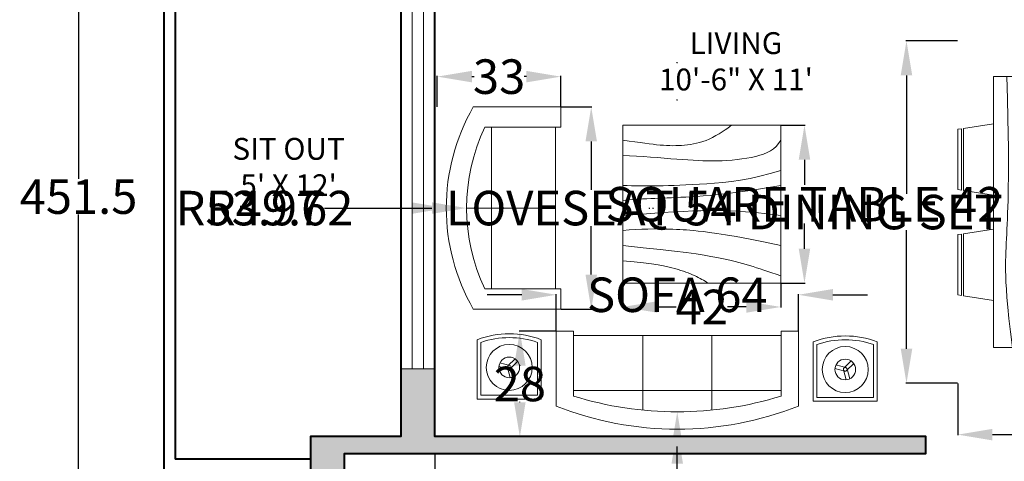
# Model space of a CAD drawing. Units: inches. Extents: x -51 to 563, y -59 to 453.
# Tile 2 of 6: x -51 to 211, y 125 to 242. Entities that reach past the tile are written whole.
import ezdxf

# ---------------------------------------------------------------- set-up
doc = ezdxf.new("R2010")
doc.units = ezdxf.units.IN
doc.header["$MEASUREMENT"] = 0
for name, color, linetype, lineweight in [('A-ANNO-DIMS', 2, 'Continuous', 18), ('A-AREA-IDEN', 7, 'Continuous', 25), ('A-FLOR-CASE', 8, 'Continuous', 25), ('A-FURN', 8, 'Continuous', 18), ('A-GLAZ', 4, 'Continuous', 18), ('A-WALL', 7, 'Continuous', 40), ('A-WALL-PATT', 252, 'Continuous', 13)]:
    doc.layers.add(name, color=color, linetype=linetype, lineweight=lineweight)
doc.styles.get("Standard").update_dxf_attribs({"font": 'arial.ttf'})
doc.dimstyles.get("Standard").update_dxf_attribs({"dimtxt": 9.18, "dimasz": 9.18, "dimexe": 0.18, "dimexo": 0.0625, "dimgap": 0.09, "dimtad": 0, "dimtih": 1, "dimtoh": 1, "dimdec": 1, "dimzin": 0, "dimdsep": 46, "dimlunit": 3, "dimtxsty": 'Standard', "dimcen": 0.09, "dimadec": 0, "dimazin": 0, "dimtfac": 1, "dimtdec": 1, "dimtofl": 0, "dimtmove": 0, "dimatfit": 3, "dimfxl": 1, "dimtolj": 1, "dimtzin": 0, "dimarcsym": 0})

# ---------------------------------------------------------------- blocks, each defined once
blk = doc.blocks.new('Dining Set - 36 x 72 in.')
for p, q in [((-22, 27.5), (-22.1562, 26.50042)), ((-5.8416, 26.5), (-22.1534, 26.5)), ((-22, 27.5), (-6, 27.5)), ((-5.8437, 26.49966), (-6, 27.5)), ((6, 27.5), (5.8438, 26.50042)), ((22.1584, 26.5), (5.8466, 26.5)), ((6, 27.5), (22, 27.5)), ((22.1563, 26.49966), (22, 27.5)), ((-22.2343, 26.00059), (-23.4847, 17.99762)), ((-22.2304, 26), (-5.7608, 26)), ((-4.5152, 17.99762), (-5.7655, 25.99926)), ((5.7657, 26.00059), (4.5153, 17.99762)), ((5.7696, 26), (22.2392, 26)), ((23.4848, 17.99762), (22.2345, 25.99926)), ((36, 18), (-36, 18)), ((-36, 18), (-36, -18)), ((36, -18), (36, 18)), ((-45.5, 8), (-44.5004, 8.15617)), ((-45.5, 8), (-45.5, -8)), ((-44.5, -8.15843), (-44.5, 8.15338)), ((-44.0006, 8.23428), (-35.9976, 9.48474)), ((-44, 8.23041), (-44, -8.23915)), ((44.0006, 8.23428), (35.9976, 9.48474)), ((44, 8.23041), (44, -8.23915)), ((44.5, -8.15843), (44.5, 8.15338)), ((45.5, 8), (44.5005, 8.15617)), ((45.5, 8), (45.5, -8)), ((-44.4997, -8.15631), (-45.5, -8)), ((-35.9976, -9.48476), (-43.9993, -8.2345)), ((35.9976, -9.48476), (43.9993, -8.2345)), ((44.4997, -8.15631), (45.5, -8)), ((-36, -18), (36, -18)), ((-22.2343, -26.0006), (-23.4847, -17.99762)), ((-4.5152, -17.99762), (-5.7655, -25.99928)), ((5.7657, -26.0006), (4.5153, -17.99762)), ((23.4848, -17.99762), (22.2345, -25.99928)), ((-22.2304, -26), (-5.7608, -26)), ((5.7696, -26), (22.2392, -26)), ((-22, -27.5), (-22.1562, -26.50044)), ((-5.8416, -26.5), (-22.1534, -26.5)), ((-22, -27.5), (-6, -27.5)), ((-5.8437, -26.49967), (-6, -27.5)), ((6, -27.5), (5.8438, -26.50044)), ((22.1584, -26.5), (5.8466, -26.5)), ((6, -27.5), (22, -27.5)), ((22.1563, -26.49967), (22, -27.5))]:
    blk.add_line(p, q)
for points in [[(-36, 15), (-31.1772, 14.97754), (-26.8079, 14.91406), (-22.8538, 14.81543), (-19.276, 14.6875), (-16.0362, 14.53613), (-13.0957, 14.36718), (-10.4159, 14.18652), (-7.9583, 14), (-5.6904, 13.81315), (-3.6035, 13.63021), (-1.6954, 13.45508), (0.0365, 13.29166), (1.5945, 13.14388), (2.9811, 13.01562), (4.1988, 12.9108), (5.25, 12.83333), (6.1393, 12.78613), (6.8802, 12.76823), (7.4883, 12.77767), (7.9792, 12.8125), (8.3685, 12.87077), (8.6719, 12.95052), (8.9049, 13.0498), (9.0833, 13.16666), (9.2205, 13.29899), (9.3216, 13.44401), (9.3895, 13.59879), (9.4271, 13.76041), (9.4373, 13.92594), (9.4232, 14.09245), (9.3875, 14.257), (9.3333, 14.41666), (9.2638, 14.56917), (9.1836, 14.71484), (9.0975, 14.85465), (9.0104, 14.98958), (8.9272, 15.1206), (8.8529, 15.2487), (8.7922, 15.37483), (8.75, 15.5), (8.7305, 15.62467), (8.7344, 15.74739), (8.7617, 15.86621), (8.8125, 15.97916), (8.8867, 16.08431), (8.9844, 16.17968), (9.1055, 16.26334), (9.25, 16.33333), (9.4189, 16.38802), (9.6172, 16.42708), (9.8506, 16.45052), (10.125, 16.45833), (10.4463, 16.45052), (10.8203, 16.42708), (11.2529, 16.38802), (11.75, 16.33333), (12.3184, 16.26318), (12.9694, 16.17838), (13.7151, 16.07991), (14.5677, 15.96875), (15.5395, 15.84586), (16.6426, 15.71224), (17.8893, 15.56884), (19.2917, 15.41666), (20.859, 15.25667), (22.5879, 15.08984), (24.4721, 14.91715), (26.5052, 14.73958), (28.6809, 14.5581), (30.9929, 14.3737), (33.4347, 14.18733), (36, 14)], [(-36, 10), (-28.9766, 10.14274), (-23.1725, 10.20442), (-18.4241, 10.19775), (-14.5677, 10.13541), (-11.4399, 10.03011), (-8.877, 9.89453), (-6.7154, 9.74137), (-4.7917, 9.58333), (-2.9698, 9.43082), (-1.2246, 9.28515), (0.4415, 9.14534), (2.026, 9.01041), (3.5266, 8.87939), (4.9408, 8.7513), (6.266, 8.62516), (7.5, 8.5), (8.6411, 8.37549), (9.6914, 8.2539), (10.6538, 8.13818), (11.5312, 8.03125), (12.3267, 7.93603), (13.043, 7.85547), (13.6831, 7.79248), (14.25, 7.75), (14.7471, 7.7303), (15.1797, 7.73307), (15.5537, 7.75732), (15.875, 7.80208), (16.1494, 7.86637), (16.3828, 7.94922), (16.5811, 8.04964), (16.75, 8.16666), (16.8944, 8.29915), (17.0143, 8.44531), (17.1089, 8.60319), (17.1771, 8.77083), (17.218, 8.94629), (17.2305, 9.1276), (17.2137, 9.31282), (17.1667, 9.5), (17.0895, 9.6875), (16.987, 9.875), (16.8649, 10.0625), (16.7292, 10.25), (16.5856, 10.4375), (16.4401, 10.625), (16.2985, 10.8125), (16.1667, 11), (16.05, 11.18733), (15.9518, 11.3737), (15.8752, 11.5581), (15.8229, 11.73958), (15.798, 11.91715), (15.8034, 12.08984), (15.842, 12.25667), (15.9167, 12.41666), (16.0295, 12.56836), (16.1784, 12.70833), (16.3605, 12.83268), (16.5729, 12.9375), (16.8127, 13.01888), (17.0768, 13.07291), (17.3625, 13.0957), (17.6667, 13.08333), (17.9894, 13.03312), (18.3418, 12.94726), (18.7382, 12.82918), (19.1927, 12.68229), (19.7195, 12.51001), (20.3327, 12.31575), (21.0465, 12.10294), (21.875, 11.875), (22.8357, 11.63354), (23.959, 11.37304), (25.2786, 11.08618), (26.8282, 10.76562), (28.6414, 10.40405), (30.752, 9.99414), (33.1936, 9.52856), (36, 9)], [(-36, 5.5), (-30.7157, 5.3348), (-26.069, 5.20963), (-21.9946, 5.11767), (-18.4271, 5.05208), (-15.3009, 5.00602), (-12.5508, 4.97265), (-10.1112, 4.94515), (-7.9167, 4.91666), (-5.909, 4.88167), (-4.0586, 4.83984), (-2.3429, 4.79215), (-0.7396, 4.73958), (0.7739, 4.6831), (2.22, 4.6237), (3.6213, 4.56233), (5, 4.5), (6.373, 4.43782), (7.7344, 4.3776), (9.0723, 4.32129), (10.375, 4.27083), (11.6309, 4.22819), (12.8281, 4.19531), (13.9551, 4.17415), (15, 4.16666), (15.954, 4.17448), (16.819, 4.19791), (17.6001, 4.23698), (18.3021, 4.29166), (18.9299, 4.36198), (19.4883, 4.44791), (19.9823, 4.54948), (20.4167, 4.66666), (20.7969, 4.79899), (21.1302, 4.94401), (21.4245, 5.09879), (21.6875, 5.26041), (21.9271, 5.42594), (22.1511, 5.59245), (22.3672, 5.757), (22.5834, 5.91666), (22.8065, 6.06868), (23.0404, 6.21093), (23.2879, 6.34147), (23.5521, 6.45833), (23.8358, 6.55957), (24.142, 6.64323), (24.4735, 6.70735), (24.8334, 6.75), (25.2235, 6.76969), (25.642, 6.76692), (26.0858, 6.74267), (26.5521, 6.69791), (27.0379, 6.63362), (27.5404, 6.55078), (28.0565, 6.45036), (28.5834, 6.33333), (29.1242, 6.19987), (29.7071, 6.04687), (30.3661, 5.87044), (31.1354, 5.66666), (32.0493, 5.43164), (33.142, 5.16146), (34.4475, 4.85221), (36, 4.5)], [(-36, -1), (-30.7915, -0.6591), (-26.0195, -0.38216), (-21.6519, -0.16284), (-17.6563, 0.00521), (-14.0005, 0.12833), (-10.6523, 0.21289), (-7.5796, 0.26522), (-4.75, 0.29166), (-2.134, 0.29793), (0.2878, 0.28711), (2.5317, 0.26163), (4.6146, 0.22396), (6.5529, 0.17651), (8.3633, 0.12174), (10.0623, 0.06209), (11.6667, 0), (13.1899, -0.06201), (14.6341, -0.1211), (15.9982, -0.17432), (17.2813, -0.21875), (18.4823, -0.25147), (19.6003, -0.26953), (20.6343, -0.27002), (21.5834, -0.25), (22.4481, -0.20768), (23.2357, -0.14584), (23.9549, -0.06836), (24.6146, 0.02083), (25.2235, 0.11784), (25.7904, 0.21875), (26.3241, 0.31966), (26.8334, 0.41666), (27.3265, 0.50618), (27.8099, 0.58593), (28.2894, 0.65397), (28.7709, 0.70833), (29.2601, 0.74707), (29.763, 0.76823), (30.2855, 0.76985), (30.8334, 0.75), (31.4088, 0.70784), (31.9994, 0.64713), (32.589, 0.57275), (33.1615, 0.48958), (33.7008, 0.4025), (34.1908, 0.3164), (34.6153, 0.23616), (34.9584, 0.16666), (35.2099, 0.11165), (35.3848, 0.07031), (35.504, 0.04069), (35.5886, 0.02083), (35.6594, 0.00879), (35.7377, 0.0026), (35.8442, 0.00032), (36, 0)], [(-36, -6.5), (-27.1843, -6.31267), (-20.084, -6.1263), (-14.469, -5.9419), (-10.1094, -5.76042), (-6.7752, -5.58285), (-4.2363, -5.41016), (-2.2629, -5.24333), (-0.625, -5.08334), (0.8708, -4.93099), (2.2715, -4.78646), (3.5872, -4.64974), (4.8281, -4.52084), (6.0046, -4.39974), (7.127, -4.28646), (8.2053, -4.18099), (9.25, -4.08334), (10.2705, -3.99382), (11.2734, -3.91407), (12.2647, -3.84603), (13.25, -3.79167), (14.2354, -3.75293), (15.2266, -3.73177), (16.2295, -3.73015), (17.25, -3.75), (18.2912, -3.79248), (19.3451, -3.85547), (20.4009, -3.93604), (21.4479, -4.03125), (22.4754, -4.13819), (23.4727, -4.25391), (24.4289, -4.37549), (25.3334, -4.5), (26.1785, -4.62492), (26.9694, -4.74935), (27.7145, -4.87281), (28.4219, -4.99479), (29.1, -5.11483), (29.7572, -5.23242), (30.4016, -5.34709), (31.0417, -5.45834), (31.6837, -5.56437), (32.3262, -5.65821), (32.9658, -5.73153), (33.599, -5.77604), (34.2224, -5.78345), (34.8327, -5.74545), (35.4264, -5.65373), (36, -5.5)], [(-36, -10), (-26.4022, -9.81299), (-18.4675, -9.62891), (-11.9839, -9.45069), (-6.7396, -9.28125), (-2.5226, -9.12354), (0.8789, -8.98047), (3.6769, -8.85498), (6.0833, -8.75), (8.2767, -8.66765), (10.3021, -8.60677), (12.1712, -8.56543), (13.8958, -8.54167), (15.4876, -8.53353), (16.9583, -8.53907), (18.3197, -8.55632), (19.5834, -8.58334), (20.7616, -8.61841), (21.8685, -8.66081), (22.9188, -8.71004), (23.9271, -8.76563), (24.9081, -8.82707), (25.8763, -8.89388), (26.8465, -8.96558), (27.8334, -9.04167), (28.8474, -9.12118), (29.8828, -9.20117), (30.93, -9.27824), (31.9792, -9.34896), (33.0205, -9.40991), (34.0443, -9.45768), (35.0407, -9.48885), (36, -9.5)], [(-36, -14.5), (-30.0881, -14.33513), (-25.0332, -14.21224), (-20.7312, -14.12647), (-17.0781, -14.07292), (-13.97, -14.04671), (-11.3027, -14.04297), (-8.9724, -14.05681), (-6.875, -14.08334), (-4.9224, -14.11833), (-3.0905, -14.16016), (-1.3709, -14.20785), (0.2448, -14.26042), (1.7647, -14.3169), (3.1973, -14.3763), (4.5507, -14.43767), (5.8333, -14.5), (7.0554, -14.5621), (8.235, -14.62175), (9.3922, -14.67652), (10.5469, -14.72396), (11.7192, -14.76164), (12.929, -14.78711), (14.1965, -14.79794), (15.5417, -14.79167), (16.9933, -14.76424), (18.6152, -14.70508), (20.4804, -14.60197), (22.6615, -14.44271), (25.2312, -14.21509), (28.2624, -13.9069), (31.8277, -13.50594), (36, -13)]]:
    blk.add_lwpolyline(points)
blk = doc.blocks.new('Sofa - Roundback 7 ft.')
for p, q in [((-12.00002, -32.4421), (-12.00003, -6.5971)), ((11.99997, -32.4421), (11.99998, -6.5971)), ((-36.000027, -34), (-36.000027, -11.4696)), ((-35.999844, -13.3819), (35.9998, -13.3819)), ((35.99998, -34), (35.99998, -11.4696)), ((-36.000027, -32.4421), (35.99998, -32.4421))]:
    blk.add_line(p, q)
for points in [[(-36.000027, -34), (-42.000027, -34), (-42.000027, -8)], [(41.99998, -8), (41.99998, -34), (35.99998, -34)]]:
    blk.add_lwpolyline(points)
for centre, radius, start, end in [((0, -114.25), 114.25, 68.43141, 111.5686), ((-0.00001, -127.1968), 121.1968, 72.72033, 107.2797)]:
    blk.add_arc(centre, radius, start, end)
blk = doc.blocks.new('Sofa - Roundback Loveseat 5 ft.')
for p, q in [((0, -32.44198), (0, -5.99998)), ((-24, -33.99998), (-24, -11.46958)), ((24.00004, -33.99998), (24.00004, -11.46958)), ((-23.9998, -13.38178), (23.99986, -13.38178)), ((-24, -32.44198), (24.00004, -32.44198))]:
    blk.add_line(p, q)
for points in [[(-24, -33.99998), (-30, -33.99998), (-30, -7.99998)], [(30.00004, -7.99998), (30.00004, -33.99998), (24.00004, -33.99998)]]:
    blk.add_lwpolyline(points)
for centre, radius, start, end in [((0, -60.24998), 60.24998, 60.13715, 119.8628), ((0, -61.38438), 55.38444, 64.32083, 115.6792)]:
    blk.add_arc(centre, radius, start, end)
blk = doc.blocks.new('Table - Square Woodgrain 42 x 42 in.')
blk.add_line((0, -42), (42, -42))
for points in [[(0, -4), (1.704, -4.2172), (3.2358, -4.4188), (4.615, -4.604), (5.8615, -4.7721), (6.9951, -4.9224), (8.0357, -5.0541), (9.0031, -5.1667), (9.9171, -5.2594), (10.7951, -5.3316), (11.6445, -5.3836), (12.4702, -5.4157), (13.277, -5.4283), (14.0698, -5.4217), (14.8535, -5.3964), (15.6331, -5.3526), (16.4133, -5.2908), (17.1986, -5.2103), (17.9913, -5.1062), (18.793, -4.9727), (19.6056, -4.8038), (20.4307, -4.5937), (21.2701, -4.3365), (22.1256, -4.0262), (22.9989, -3.6571), (23.888, -3.2272), (24.7756, -2.7516), (25.6408, -2.2491), (26.4624, -1.7387), (27.2195, -1.2395), (27.891, -0.7703), (28.456, -0.3501), (28.8934, 0.002)], [(0, -42), (0, 0), (42, 0), (42, -42)], [(0, -8), (1.8203, -8.1001), (3.6741, -8.2149), (5.5411, -8.3408), (7.4011, -8.4741), (9.2339, -8.6112), (11.0193, -8.7484), (12.7371, -8.8821), (14.3671, -9.0086), (15.8954, -9.1246), (17.3337, -9.2278), (18.6997, -9.3159), (20.0116, -9.387), (21.2871, -9.4389), (22.5442, -9.4696), (23.8008, -9.477), (25.0749, -9.459), (26.3791, -9.4137), (27.7049, -9.3403), (29.0383, -9.2382), (30.3655, -9.1068), (31.6728, -8.9455), (32.9461, -8.7535), (34.1717, -8.5304), (35.3358, -8.2756), (36.4268, -7.9863), (37.443, -7.6521), (38.3849, -7.2603), (39.253, -6.7986), (40.048, -6.2542), (40.7705, -5.6147), (41.421, -4.8674), (42, -4)], [(42, -12), (39.1784, -12.8621), (36.4519, -13.5654), (33.8246, -14.1294), (31.3004, -14.5731), (28.8832, -14.9161), (26.577, -15.1775), (24.3858, -15.3768), (22.3136, -15.5332), (20.3622, -15.6632), (18.5254, -15.7718), (16.7947, -15.8612), (15.1618, -15.9338), (13.6183, -15.9916), (12.1558, -16.0369), (10.7659, -16.0718), (9.4403, -16.0987), (8.1703, -16.1191), (6.9461, -16.1325), (5.7577, -16.1377), (4.595, -16.1335), (3.4479, -16.1188), (2.3064, -16.0924), (1.1604, -16.0532), (0, -16)], [(42, -16), (37.6529, -16.7365), (33.8802, -17.329), (30.6179, -17.7961), (27.8015, -18.1561), (25.3668, -18.4275), (23.2497, -18.6288), (21.3859, -18.7785), (19.7111, -18.8949), (18.1693, -18.9939), (16.7375, -19.0795), (15.401, -19.1534), (14.1449, -19.217), (12.9544, -19.2717), (11.8148, -19.3191), (10.7113, -19.3606), (9.6291, -19.3976), (8.5534, -19.4323), (7.47, -19.4689), (6.3643, -19.5122), (5.222, -19.5672), (4.0288, -19.6386), (2.7703, -19.7313), (1.4321, -19.8501), (0, -20)], [(0, -24), (3.9243, -23.6805), (7.4766, -23.4138), (10.6891, -23.1954), (13.5943, -23.0205), (16.2247, -22.8847), (18.6125, -22.7832), (20.7903, -22.7116), (22.7903, -22.6651), (24.6563, -22.642), (26.4764, -22.6507), (28.35, -22.7024), (30.3766, -22.8084), (32.6555, -22.98), (35.2861, -23.2283), (38.3678, -23.5645), (42, -24)], [(42, -32), (37.392, -31.017), (33.4585, -30.2231), (30.1291, -29.5949), (27.3334, -29.109), (25.0009, -28.742), (23.0612, -28.4707), (21.4439, -28.2716), (20.0786, -28.1215), (18.8998, -28.0002), (17.8609, -27.9014), (16.9206, -27.8219), (16.0371, -27.7588), (15.1691, -27.709), (14.2748, -27.6693), (13.3128, -27.6368), (12.2415, -27.6083), (11.0295, -27.5824), (9.6867, -27.5643), (8.233, -27.5608), (6.6884, -27.5787), (5.0728, -27.6248), (3.4062, -27.7058), (1.7086, -27.8286), (0, -28)], [(0, -32), (5.4026, -32.5358), (9.9494, -33.019), (13.7424, -33.4553), (16.8834, -33.8505), (19.4743, -34.2106), (21.6171, -34.5413), (23.4136, -34.8486), (24.9657, -35.1382), (26.3614, -35.4156), (27.6332, -35.6841), (28.7995, -35.9467), (29.8788, -36.2064), (30.8897, -36.4661), (31.8507, -36.7288), (32.7802, -36.9973), (33.6968, -37.2747), (34.6175, -37.5635), (35.5531, -37.8651), (36.5128, -38.1805), (37.506, -38.5108), (38.5421, -38.8568), (39.6302, -39.2197), (40.7797, -39.6004), (42, -40)], [(0, -36), (3.0098, -36.2857), (5.5354, -36.5643), (7.6368, -36.8359), (9.374, -37.1009), (10.807, -37.3597), (11.9957, -37.6126), (13.0002, -37.8599), (13.8804, -38.102), (14.6874, -38.3393), (15.4365, -38.5729), (16.1338, -38.8041), (16.7858, -39.0341), (17.3987, -39.264), (17.9787, -39.4952), (18.5322, -39.7288), (19.0655, -39.9662), (19.5832, -40.2081), (20.0842, -40.4544), (20.5657, -40.7046), (21.0249, -40.9581), (21.459, -41.2144), (21.8653, -41.4731), (22.2409, -41.7335), (22.5831, -41.9951)]]:
    blk.add_lwpolyline(points)
blk = doc.blocks.new('*U11')
for p, q in [((-1.31, -0.61), (0.61, 1.31)), ((-0.61, -1.31), (1.31, 0.61))]:
    blk.add_line(p, q)
blk = doc.blocks.new('*U12')
at = {"color": 0, "linetype": 'ByBlock', "lineweight": -2, "transparency": 16777216}
for p, rotation in [((276.07, -10.08), 120), ((277.73, -11.74), 239.9999999999999)]:
    blk.add_blockref('*U11', p, dxfattribs=dict(at, rotation=rotation))
blk.add_blockref('*U11', (278.34, -9.47), dxfattribs=at)
blk = doc.blocks.new('TABLE-SIDE-WITH-LAMP')
for points in [[(17.03, 15.79), (17.03, 0), (0, 0), (0, 15.79, -0.18199)], [(16.03, 15.08), (16.03, 1), (1, 1), (1, 15.08, -0.16668)]]:
    blk.add_lwpolyline(points, format="xyb", close=True)
for centre, radius in [((8.51, 8.42), 6.11), ((8.51, 8.42), 2.75), ((8.51, 8.47), 0.5)]:
    blk.add_circle(centre, radius)
blk.add_blockref('*U12', (-268.87, 18.9))
blk = doc.blocks.new('*D31')
at = {"layer": 'A-ANNO-DIMS', "color": 0, "lineweight": -2, "transparency": 16777216}
for p, q in [((93.14, 218.93), (101.32, 218.93)), ((101.14, 209.75), (101.14, 196.89)), ((101.14, 174.36), (101.14, 187.21)), ((93.14, 165.18), (101.32, 165.18))]:
    blk.add_line(p, q, dxfattribs=at)
at = {"layer": 'A-ANNO-DIMS', "color": 0, "transparency": 16777216}
for points in [[(99.61, 209.75), (102.67, 209.75), (101.14, 218.93)], [(99.61, 174.36), (102.67, 174.36), (101.14, 165.18)]]:
    blk.add_solid(points, dxfattribs=at)
at = {"layer": 'Defpoints', "color": 0, "transparency": 16777216}
for p in [(93.07, 218.93), (101.14, 218.93), (93.07, 165.18)]:
    blk.add_point(p, dxfattribs=at)
at = {"layer": 'A-ANNO-DIMS', "color": 0, "transparency": 16777216, "insert": (101.14, 192.05), "char_height": 9.18, "attachment_point": 5}
blk.add_mtext('\\A1;LOVESEAT 54', dxfattribs=at)
blk = doc.blocks.new('*D32')
at = {"layer": 'A-ANNO-DIMS', "color": 0, "lineweight": -2, "transparency": 16777216}
for p, q in [((60.23, 218.99), (60.23, 227.17)), ((69.41, 226.99), (69.99, 226.99)), ((83.89, 226.99), (83.31, 226.99)), ((93.07, 218.99), (93.07, 227.17))]:
    blk.add_line(p, q, dxfattribs=at)
at = {"layer": 'A-ANNO-DIMS', "color": 0, "transparency": 16777216}
for points in [[(69.41, 228.52), (69.41, 225.46), (60.23, 226.99)], [(83.89, 228.52), (83.89, 225.46), (93.07, 226.99)]]:
    blk.add_solid(points, dxfattribs=at)
at = {"layer": 'Defpoints', "color": 0, "transparency": 16777216}
for p in [(60.23, 226.99), (60.23, 218.93), (93.07, 218.93)]:
    blk.add_point(p, dxfattribs=at)
at = {"layer": 'A-ANNO-DIMS', "color": 0, "transparency": 16777216, "insert": (76.65, 226.99), "char_height": 9.18, "attachment_point": 5}
blk.add_mtext('\\A1;33', dxfattribs=at)
blk = doc.blocks.new('*D37')
at = {"layer": 'A-ANNO-DIMS', "color": 0, "lineweight": -2, "transparency": 16777216}
for p, q in [((82.65, 169.01), (73.47, 169.01)), ((91.83, 159.41), (91.83, 169.19)), ((156.2, 159.41), (156.2, 169.19)), ((165.38, 169.01), (174.56, 169.01))]:
    blk.add_line(p, q, dxfattribs=at)
at = {"layer": 'A-ANNO-DIMS', "color": 0, "transparency": 16777216}
for points in [[(82.65, 170.54), (82.65, 167.48), (91.83, 169.01)], [(165.38, 170.54), (165.38, 167.48), (156.2, 169.01)]]:
    blk.add_solid(points, dxfattribs=at)
at = {"layer": 'Defpoints', "color": 0, "transparency": 16777216}
for p in [(91.83, 169.01), (91.83, 159.35), (156.2, 159.35)]:
    blk.add_point(p, dxfattribs=at)
at = {"layer": 'A-ANNO-DIMS', "color": 0, "transparency": 16777216, "insert": (124.01, 169.01), "char_height": 9.18, "attachment_point": 5}
blk.add_mtext('\\A1;SOFA 64', dxfattribs=at)
blk = doc.blocks.new('*D38')
at = {"layer": 'A-ANNO-DIMS', "color": 0, "lineweight": -2, "transparency": 16777216}
for p, q in [((91.76, 159.35), (81.99, 159.35)), ((82.17, 150.17), (82.17, 150.08)), ((82.17, 140.43), (82.17, 140.52)), ((91.76, 131.25), (81.99, 131.25))]:
    blk.add_line(p, q, dxfattribs=at)
at = {"layer": 'A-ANNO-DIMS', "color": 0, "transparency": 16777216}
for points in [[(80.64, 150.17), (83.7, 150.17), (82.17, 159.35)], [(80.64, 140.43), (83.7, 140.43), (82.17, 131.25)]]:
    blk.add_solid(points, dxfattribs=at)
at = {"layer": 'Defpoints', "color": 0, "transparency": 16777216}
for p in [(91.83, 159.35), (82.17, 131.25), (91.83, 131.25)]:
    blk.add_point(p, dxfattribs=at)
at = {"layer": 'A-ANNO-DIMS', "color": 0, "transparency": 16777216, "insert": (82.17, 145.3), "char_height": 9.18, "attachment_point": 5}
blk.add_mtext('\\A1;28', dxfattribs=at)
blk = doc.blocks.new('*D50')
at = {"layer": 'A-ANNO-DIMS', "color": 0, "lineweight": -2, "transparency": 16777216}
for p, q in [((217.6, 120.04), (208.42, 120.04)), ((226.78, 117.06), (226.78, 120.22)), ((243.37, 117.06), (243.37, 120.22)), ((252.55, 120.04), (261.73, 120.04))]:
    blk.add_line(p, q, dxfattribs=at)
at = {"layer": 'A-ANNO-DIMS', "color": 0, "transparency": 16777216}
for points in [[(217.6, 121.57), (217.6, 118.51), (226.78, 120.04)], [(252.55, 121.57), (252.55, 118.51), (243.37, 120.04)]]:
    blk.add_solid(points, dxfattribs=at)
at = {"layer": 'Defpoints', "color": 0, "transparency": 16777216}
for p in [(226.78, 120.04), (226.78, 117), (243.37, 117)]:
    blk.add_point(p, dxfattribs=at)
at = {"layer": 'A-ANNO-DIMS', "color": 0, "transparency": 16777216, "insert": (235.08, 120.04), "char_height": 9.18, "attachment_point": 5}
blk.add_mtext('\\A1;17', dxfattribs=at)
blk = doc.blocks.new('*D57')
at = {"layer": 'A-ANNO-DIMS', "color": 0, "lineweight": -2, "transparency": 16777216}
for p, q in [((198.52, 236.49), (184.76, 236.49)), ((184.94, 227.31), (184.94, 195.82)), ((184.94, 154.67), (184.94, 186.15)), ((198.52, 145.49), (184.76, 145.49))]:
    blk.add_line(p, q, dxfattribs=at)
at = {"layer": 'A-ANNO-DIMS', "color": 0, "transparency": 16777216}
for points in [[(183.41, 227.31), (186.47, 227.31), (184.94, 236.49)], [(183.41, 154.67), (186.47, 154.67), (184.94, 145.49)]]:
    blk.add_solid(points, dxfattribs=at)
at = {"layer": 'Defpoints', "color": 0, "transparency": 16777216}
for p in [(198.59, 236.49), (184.94, 145.49), (198.59, 145.49)]:
    blk.add_point(p, dxfattribs=at)
at = {"layer": 'A-ANNO-DIMS', "color": 0, "transparency": 16777216, "insert": (184.94, 190.99), "char_height": 9.18, "attachment_point": 5}
blk.add_mtext('\\A1;DINING SET 91', dxfattribs=at)
blk = doc.blocks.new('*D58')
at = {"layer": 'A-ANNO-DIMS', "color": 0, "lineweight": -2, "transparency": 16777216}
for p, q in [((198.59, 145.43), (198.59, 131.66)), ((253.59, 145.43), (253.59, 131.66)), ((207.77, 131.84), (219.39, 131.84)), ((244.41, 131.84), (232.79, 131.84))]:
    blk.add_line(p, q, dxfattribs=at)
at = {"layer": 'A-ANNO-DIMS', "color": 0, "transparency": 16777216}
for points in [[(207.77, 133.37), (207.77, 130.31), (198.59, 131.84)], [(244.41, 133.37), (244.41, 130.31), (253.59, 131.84)]]:
    blk.add_solid(points, dxfattribs=at)
at = {"layer": 'Defpoints', "color": 0, "transparency": 16777216}
for p in [(198.59, 145.49), (253.59, 145.49), (253.59, 131.84)]:
    blk.add_point(p, dxfattribs=at)
at = {"layer": 'A-ANNO-DIMS', "color": 0, "transparency": 16777216, "insert": (226.09, 131.84), "char_height": 9.18, "attachment_point": 5}
blk.add_mtext('\\A1;55', dxfattribs=at)
blk = doc.blocks.new('*D59')
at = {"layer": 'A-ANNO-DIMS', "color": 0, "lineweight": -2, "transparency": 16777216}
for p, q in [((151.59, 214.07), (158, 214.07)), ((157.82, 204.89), (157.82, 198.19)), ((157.82, 181.25), (157.82, 187.95)), ((151.59, 172.07), (158, 172.07))]:
    blk.add_line(p, q, dxfattribs=at)
at = {"layer": 'A-ANNO-DIMS', "color": 0, "transparency": 16777216}
for points in [[(156.29, 204.89), (159.35, 204.89), (157.82, 214.07)], [(156.29, 181.25), (159.35, 181.25), (157.82, 172.07)]]:
    blk.add_solid(points, dxfattribs=at)
at = {"layer": 'Defpoints', "color": 0, "transparency": 16777216}
for p in [(151.52, 214.07), (157.82, 214.07), (151.52, 172.07)]:
    blk.add_point(p, dxfattribs=at)
at = {"layer": 'A-ANNO-DIMS', "color": 0, "transparency": 16777216, "insert": (157.82, 193.07), "char_height": 9.18, "attachment_point": 5}
blk.add_mtext('\\A1;SQUARE TABLE 42', dxfattribs=at)
blk = doc.blocks.new('*D60')
at = {"layer": 'A-ANNO-DIMS', "color": 0, "lineweight": -2, "transparency": 16777216}
for p, q in [((109.52, 172), (109.52, 165.59)), ((151.52, 172), (151.52, 165.59)), ((118.7, 165.77), (123.72, 165.77)), ((142.34, 165.77), (137.33, 165.77))]:
    blk.add_line(p, q, dxfattribs=at)
at = {"layer": 'A-ANNO-DIMS', "color": 0, "transparency": 16777216}
for points in [[(118.7, 167.3), (118.7, 164.24), (109.52, 165.77)], [(142.34, 167.3), (142.34, 164.24), (151.52, 165.77)]]:
    blk.add_solid(points, dxfattribs=at)
at = {"layer": 'Defpoints', "color": 0, "transparency": 16777216}
for p in [(109.52, 172.07), (151.52, 172.07), (151.52, 165.77)]:
    blk.add_point(p, dxfattribs=at)
at = {"layer": 'A-ANNO-DIMS', "color": 0, "transparency": 16777216, "insert": (130.52, 165.77), "char_height": 9.18, "attachment_point": 5}
blk.add_mtext('\\A1;42', dxfattribs=at)
blk = doc.blocks.new('*D66')
at = {"layer": 'A-ANNO-DIMS', "color": 0, "lineweight": -2, "transparency": 16777216}
for p, q in [((26.5, 420.85), (-35.32, 420.85)), ((-35.14, 411.67), (-35.14, 199.87)), ((-35.14, -21.47), (-35.14, 190.32)), ((26.5, -30.65), (-35.32, -30.65))]:
    blk.add_line(p, q, dxfattribs=at)
at = {"layer": 'A-ANNO-DIMS', "color": 0, "transparency": 16777216}
for points in [[(-36.67, 411.67), (-33.61, 411.67), (-35.14, 420.85)], [(-36.67, -21.47), (-33.61, -21.47), (-35.14, -30.65)]]:
    blk.add_solid(points, dxfattribs=at)
at = {"layer": 'Defpoints', "color": 0, "transparency": 16777216}
for p in [(-35.14, 420.85), (26.56, 420.85), (26.56, -30.65)]:
    blk.add_point(p, dxfattribs=at)
at = {"layer": 'A-ANNO-DIMS', "color": 0, "transparency": 16777216, "insert": (-35.14, 195.1), "char_height": 9.18, "attachment_point": 5}
blk.add_mtext('\\A1;451.5', dxfattribs=at)
blk = doc.blocks.new('*D89')
at = {"layer": 'A-ANNO-DIMS', "color": 0, "lineweight": -2, "transparency": 16777216}
for p, q in [((123.92, 230.78), (124.1, 230.78)), ((124.01, 230.69), (124.01, 230.87)), ((124.01, 82.16), (124.01, 128.71)), ((114.83, 82.16), (124.01, 82.16))]:
    blk.add_line(p, q, dxfattribs=at)
at = {"layer": 'A-ANNO-DIMS', "color": 0, "transparency": 16777216}
blk.add_solid([(122.48, 128.71), (125.54, 128.71), (124.01, 137.89)], dxfattribs=at)
at = {"layer": 'Defpoints', "color": 0, "transparency": 16777216}
for p in [(124.01, 230.78), (124.01, 137.89)]:
    blk.add_point(p, dxfattribs=at)
at = {"layer": 'A-ANNO-DIMS', "color": 0, "transparency": 16777216, "insert": (94.85, 82.16), "char_height": 9.18, "attachment_point": 5}
blk.add_mtext('\\A1;R92.88', dxfattribs=at)
blk = doc.blocks.new('*D90')
at = {"layer": 'A-ANNO-DIMS', "color": 0, "lineweight": -2, "transparency": 16777216}
for p, q in [((123.92, 220.85), (124.1, 220.85)), ((124.01, 220.76), (124.01, 220.94)), ((124.01, 80.76), (124.01, 124.11)), ((114.83, 80.76), (124.01, 80.76))]:
    blk.add_line(p, q, dxfattribs=at)
at = {"layer": 'A-ANNO-DIMS', "color": 0, "transparency": 16777216}
blk.add_solid([(122.48, 124.11), (125.54, 124.11), (124.01, 133.29)], dxfattribs=at)
at = {"layer": 'Defpoints', "color": 0, "transparency": 16777216}
for p in [(124.01, 220.85), (124.01, 133.29)]:
    blk.add_point(p, dxfattribs=at)
at = {"layer": 'A-ANNO-DIMS', "color": 0, "transparency": 16777216, "insert": (94.86, 80.76), "char_height": 9.18, "attachment_point": 5}
blk.add_mtext('\\A1;R87.56', dxfattribs=at)
blk = doc.blocks.new('*D93')
at = {"layer": 'A-ANNO-DIMS', "color": 0, "lineweight": -2, "transparency": 16777216}
for p, q in [((30.23, 192.05), (53.44, 192.05)), ((116.5, 192.05), (116.68, 192.05)), ((116.59, 191.96), (116.59, 192.14))]:
    blk.add_line(p, q, dxfattribs=at)
at = {"layer": 'A-ANNO-DIMS', "color": 0, "transparency": 16777216}
blk.add_solid([(53.44, 193.58), (53.44, 190.52), (62.62, 192.05)], dxfattribs=at)
at = {"layer": 'Defpoints', "color": 0, "transparency": 16777216}
for p in [(62.62, 192.05), (116.59, 192.05)]:
    blk.add_point(p, dxfattribs=at)
at = {"layer": 'A-ANNO-DIMS', "color": 0, "transparency": 16777216, "insert": (10.26, 192.05), "char_height": 9.18, "attachment_point": 5}
blk.add_mtext('\\A1;R53.97', dxfattribs=at)
blk = doc.blocks.new('*D94')
at = {"layer": 'A-ANNO-DIMS', "color": 0, "lineweight": -2, "transparency": 16777216}
for p, q in [((38.22, 192.05), (58.81, 192.05)), ((117.52, 192.05), (117.7, 192.05)), ((117.61, 191.96), (117.61, 192.14))]:
    blk.add_line(p, q, dxfattribs=at)
at = {"layer": 'A-ANNO-DIMS', "color": 0, "transparency": 16777216}
blk.add_solid([(58.81, 193.58), (58.81, 190.52), (67.99, 192.05)], dxfattribs=at)
at = {"layer": 'Defpoints', "color": 0, "transparency": 16777216}
for p in [(67.99, 192.05), (117.61, 192.05)]:
    blk.add_point(p, dxfattribs=at)
at = {"layer": 'A-ANNO-DIMS', "color": 0, "transparency": 16777216, "insert": (18.3, 192.05), "char_height": 9.18, "attachment_point": 5}
blk.add_mtext('\\A1;R49.62', dxfattribs=at)

msp = doc.modelspace()

# ---------------------------------------------------------------- linework, layer by layer
at = {"layer": 'A-FLOR-CASE'}
msp.add_line((59.5584, 126.8479), (59.5584, 54.8479), dxfattribs=at)
at = {"layer": 'A-GLAZ'}
for p, q in [((53.5584, 245.3479), (53.5584, 149.3479)), ((56.5584, 245.3479), (56.5584, 149.3479)), ((50.5584, 149.3479), (59.5584, 149.3479))]:
    msp.add_line(p, q, dxfattribs=at)
at = {"layer": 'A-WALL'}
for p in [(-9.4416, 269.3479), (26.5584, 125.3479)]:
    msp.add_line(p, (-9.4416, 125.3479), dxfattribs=at)
for points in [[(422.5584, 420.8479), (26.5584, 420.8479), (26.5584, 267.8479), (26.5584, 263.3479), (35.5584, 263.3479), (50.5584, 263.3479), (50.5584, 131.3479), (35.5584, 131.3479), (26.5584, 131.3479), (26.5584, 126.8479), (26.5584, 0.8479), (26.5584, -30.6521), (35.5584, -30.6521), (284.5584, -30.6521)], [(26.5584, 272.3479), (-9.4416, 272.3479), (-12.4416, 272.3479), (-12.4416, 267.8479), (-12.4416, 126.8479), (-12.4416, 122.3479), (-9.4416, 122.3479), (26.5584, 122.3479)], [(244.0584, 84.8479), (179.5584, 84.8479), (179.5584, 30.8479), (155.5584, 30.8479), (155.5584, 26.3479), (179.5584, 26.3479), (179.5584, -21.6521), (35.5584, -21.6521), (35.5584, 26.3479), (119.5584, 26.3479), (119.5584, 30.8479), (35.5584, 30.8479), (35.5584, 126.8479), (190.0584, 126.8479), (190.0584, 131.3479), (59.5584, 131.3479), (59.5584, 263.3479)]]:
    msp.add_lwpolyline(points, dxfattribs=at)
at = {"layer": 'A-WALL-PATT'}
for points in [[(50.5584, 149.3479), (59.5584, 149.3479), (50.5584, 131.3479), (59.5584, 131.3479)], [(190.0584, 131.3479), (190.0584, 126.8479), (26.5584, 131.3479), (35.5584, 126.8479)], [(26.5584, 131.3479), (35.5584, 126.8479), (26.5584, -30.6521), (35.5584, -21.6521)]]:
    msp.add_solid(points, dxfattribs=at)

# ---------------------------------------------------------------- block references
at = {"layer": 'A-FURN', "rotation": 270}
msp.add_blockref('Dining Set - 36 x 72 in.', (226.0874, 190.988), dxfattribs=at)
at = {"layer": 'A-FURN'}
for name, p, xscale, yscale, zscale, rotation in [('Sofa - Roundback Loveseat 5 ft.', (62.6163, 192.0501), 0.8958343359602521, 0.8958343359602521, 0.8958343359602521, 89.99999999999999), ('Sofa - Roundback 7 ft.', (124.0132, 133.2945), 0.7663813717622041, 0.7663813717622041, 0.7663813717622041, 180)]:
    msp.add_blockref(name, p, dxfattribs=dict(at, xscale=xscale, yscale=yscale, zscale=zscale, rotation=rotation))
for name, p in [('Table - Square Woodgrain 42 x 42 in.', (109.5237, 214.0658)), ('TABLE-SIDE-WITH-LAMP', (70.8369, 141.2871)), ('TABLE-SIDE-WITH-LAMP', (160.1514, 140.724))]:
    msp.add_blockref(name, p, dxfattribs=at)

# ---------------------------------------------------------------- texts
at = {"layer": 'A-AREA-IDEN', "char_height": 5.8, "attachment_point": 1}
for s, width, insert in [('\\pxqc;LIVING\\P10\'-6" X 11\'', 41.537394, (118.8349, 238.7948)), ("\\pxqc;SIT OUT\\P5' X 12'", 32.369193, (4.512, 210.6922))]:
    msp.add_mtext_dynamic_manual_height_columns(s, width=width, gutter_width=1, heights=[0], dxfattribs=dict(at, insert=insert))

# ---------------------------------------------------------------- dimensions: what is measured, and where the dimension line sits
at = {"layer": 'A-ANNO-DIMS'}
for base, p1, p2, angle, override, picture, middle in [((-35.1416, 420.8479), (26.5584, -30.6521), (26.5584, 420.8479), 90, {"dimdec": 1, "dimlfac": 1, "dimrnd": 0, "dimzin": 0, "dimdsep": 46, "dimlunit": 2}, '*D66', (-35.1416, 195.0979)), ((60.2274, 226.9876), (93.0747, 218.9251), (60.2274, 218.9251), 180, {"dimdec": 0, "dimlfac": 1, "dimrnd": 0, "dimzin": 0, "dimdsep": 46, "dimlunit": 2}, '*D32', (76.651, 226.9876)), ((82.1688, 131.2508), (91.8252, 159.3515), (91.8252, 131.2508), 270, {"dimdec": 0, "dimlfac": 1, "dimrnd": 0, "dimzin": 0, "dimdsep": 46, "dimlunit": 2}, '*D38', (82.1688, 145.3011)), ((226.7786, 120.0365), (243.3723, 117.0018), (226.7786, 117.0018), 180, {"dimdec": 0, "dimlfac": 1, "dimrnd": 0, "dimzin": 0, "dimdsep": 46, "dimlunit": 2}, '*D50', (235.0754, 120.0365))]:
    dim = msp.add_linear_dim(base=base, p1=p1, p2=p2, angle=angle, dimstyle='Standard', override=override, dxfattribs=at)
    dim.commit()
    dim.dimension.update_dxf_attribs({"geometry": picture, "text_midpoint": middle})
for base, p1, p2, angle, text, picture, middle in [((184.9374, 145.488), (198.5874, 236.488), (198.5874, 145.488), 270, 'DINING SET <>', '*D57', (184.9374, 190.988)), ((101.1372, 218.9251), (93.0747, 165.175), (93.0747, 218.9251), 90, 'LOVESEAT <>', '*D31', (101.1372, 192.0501)), ((157.824, 214.0678), (151.5237, 172.0658), (151.5237, 214.0678), 90, 'SQUARE TABLE <>', '*D59', (157.824, 193.0668)), ((91.8252, 169.0079), (156.2012, 159.3515), (91.8252, 159.3515), 180, 'SOFA <>', '*D37', (124.0132, 169.0079))]:
    dim = msp.add_linear_dim(base=base, p1=p1, p2=p2, angle=angle, text=text, dimstyle='Standard', override={"dimdec": 0, "dimlfac": 1, "dimrnd": 0, "dimzin": 0, "dimdsep": 46, "dimlunit": 2}, dxfattribs=at)
    dim.commit()
    dim.dimension.update_dxf_attribs({"geometry": picture, "text_midpoint": middle})
for center, mpoint, picture, middle in [((124.0132, 230.7757), (124.013, 137.8928), '*D89', (94.8518, 82.163)), ((124.0132, 220.8536), (124.013, 133.2945), '*D90', (94.8644, 80.759)), ((116.5903, 192.0501), (62.6163, 192.05), '*D93', (30.2319, 192.05)), ((117.6065, 192.0501), (67.9913, 192.05), '*D94', (38.2221, 192.05))]:
    dim = msp.add_radius_dim(center=center, mpoint=mpoint, dimstyle='Standard', override={"dimdec": 2, "dimlfac": 1, "dimrnd": 0, "dimzin": 0, "dimdsep": 46, "dimlunit": 2}, dxfattribs=at)
    dim.commit()
    dim.dimension.update_dxf_attribs({"geometry": picture, "text_midpoint": middle, "dimtype": 164})
for base, p1, p2, picture, middle in [((151.5237, 165.7655), (109.5237, 172.0658), (151.5237, 172.0658), '*D60', (130.5237, 165.7655)), ((253.5874, 131.838), (198.5874, 145.488), (253.5874, 145.488), '*D58', (226.0874, 131.838))]:
    dim = msp.add_linear_dim(base=base, p1=p1, p2=p2, dimstyle='Standard', override={"dimdec": 0, "dimlfac": 1, "dimrnd": 0, "dimzin": 0, "dimdsep": 46, "dimlunit": 2}, dxfattribs=at)
    dim.commit()
    dim.dimension.update_dxf_attribs({"geometry": picture, "text_midpoint": middle})

doc.saveas('drawing.dxf')
